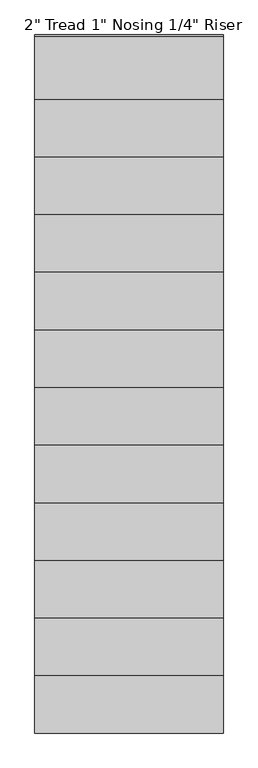
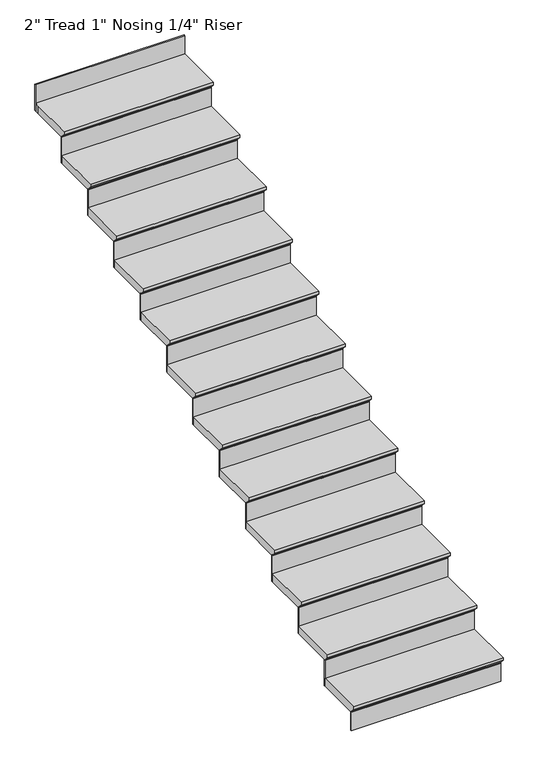
"""IFC4 building model written with IfcOpenShell, lengths in millimetres: stair flight geometry."""

from ifc_helpers import new_model, si_unit, origin, place, context, project, spatial, faceted_brep, source, transform, mapped, element, save


def stair_flight_9c09f5e7(model_context):
    return source(origin(), model_context, "Body", "Brep", [
        faceted_brep([(-2703.0415084, 19841.9216096, 37576.9005799), (-2703.0415084, 19841.9216096, 37595.9505799), (-3617.4415084, 19841.9216096, 37595.9505799), (-3617.4415084, 19841.9216096, 37576.9005799), (-2703.0415084, 19867.3216096, 37551.5005799), (-3617.4415084, 19867.3216096, 37551.5005799), (-2703.0415084, 20146.7216096, 37595.9505799), (-3617.4415084, 20146.7216096, 37595.9505799), (-3617.4415084, 19867.3216096, 37545.1505799), (-3617.4415084, 20146.7216096, 37545.1505799), (-2703.0415084, 20146.7216096, 37545.1505799), (-2703.0415084, 19867.3216096, 37545.1505799)], [[[0, 1, 2, 3]], [[4, 0, 3, 5]], [[2, 1, 6, 7]], [[8, 9, 10, 11]], [[2, 7, 9, 8, 5, 3]], [[8, 11, 4, 5]], [[6, 1, 0, 4, 11, 10]], [[7, 6, 10, 9]]]),
        faceted_brep([(-2703.0415084, 19867.3216096, 37545.1505799), (-2703.0415084, 19867.3216096, 37426.6172466), (-2703.0415084, 19873.6716096, 37426.6172466), (-2703.0415084, 19873.6716096, 37545.1505799), (-3617.4415084, 19867.3216096, 37545.1505799), (-3617.4415084, 19873.6716096, 37545.1505799), (-3617.4415084, 19873.6716096, 37426.6172466), (-3617.4415084, 19867.3216096, 37426.6172466)], [[[0, 1, 2, 3]], [[4, 5, 6, 7]], [[1, 0, 4, 7]], [[2, 1, 7, 6]], [[3, 2, 6, 5]], [[0, 3, 5, 4]]]),
        faceted_brep([(-2703.0415084, 20146.7216096, 37714.4839133), (-2703.0415084, 20146.7216096, 37545.1505799), (-2703.0415084, 20153.0716096, 37545.1505799), (-2703.0415084, 20153.0716096, 37714.4839133), (-3617.4415084, 20146.7216096, 37714.4839133), (-3617.4415084, 20153.0716096, 37714.4839133), (-3617.4415084, 20153.0716096, 37545.1505799), (-3617.4415084, 20146.7216096, 37545.1505799)], [[[0, 1, 2, 3]], [[4, 5, 6, 7]], [[1, 0, 4, 7]], [[2, 1, 7, 6]], [[3, 2, 6, 5]], [[0, 3, 5, 4]]]),
        faceted_brep([(-3617.4415084, 20121.3216096, 37765.2839133), (-2703.0415084, 20121.3216096, 37765.2839133), (-2703.0415084, 20426.1216096, 37765.2839133), (-3617.4415084, 20426.1216096, 37765.2839133), (-3617.4415084, 20146.7216096, 37714.4839133), (-3617.4415084, 20426.1216096, 37714.4839133), (-2703.0415084, 20426.1216096, 37714.4839133), (-2703.0415084, 20146.7216096, 37714.4839133), (-3617.4415084, 20146.7216096, 37720.8339133), (-3617.4415084, 20121.3216096, 37746.2339133), (-2703.0415084, 20146.7216096, 37720.8339133), (-2703.0415084, 20121.3216096, 37746.2339133)], [[[0, 1, 2, 3]], [[4, 5, 6, 7]], [[0, 3, 5, 4, 8, 9]], [[4, 7, 10, 8]], [[2, 1, 11, 10, 7, 6]], [[3, 2, 6, 5]], [[11, 1, 0, 9]], [[10, 11, 9, 8]]]),
        faceted_brep([(-2703.0415084, 20426.1216096, 37883.8172466), (-2703.0415084, 20426.1216096, 37714.4839133), (-2703.0415084, 20432.4716096, 37714.4839133), (-2703.0415084, 20432.4716096, 37883.8172466), (-3617.4415084, 20426.1216096, 37883.8172466), (-3617.4415084, 20432.4716096, 37883.8172466), (-3617.4415084, 20432.4716096, 37714.4839133), (-3617.4415084, 20426.1216096, 37714.4839133)], [[[0, 1, 2, 3]], [[4, 5, 6, 7]], [[1, 0, 4, 7]], [[2, 1, 7, 6]], [[3, 2, 6, 5]], [[0, 3, 5, 4]]]),
        faceted_brep([(-3617.4415084, 20400.7216096, 37934.6172466), (-2703.0415084, 20400.7216096, 37934.6172466), (-2703.0415084, 20705.5216096, 37934.6172466), (-3617.4415084, 20705.5216096, 37934.6172466), (-3617.4415084, 20426.1216096, 37883.8172466), (-3617.4415084, 20705.5216096, 37883.8172466), (-2703.0415084, 20705.5216096, 37883.8172466), (-2703.0415084, 20426.1216096, 37883.8172466), (-3617.4415084, 20426.1216096, 37890.1672466), (-3617.4415084, 20400.7216096, 37915.5672466), (-2703.0415084, 20426.1216096, 37890.1672466), (-2703.0415084, 20400.7216096, 37915.5672466)], [[[0, 1, 2, 3]], [[4, 5, 6, 7]], [[0, 3, 5, 4, 8, 9]], [[4, 7, 10, 8]], [[2, 1, 11, 10, 7, 6]], [[3, 2, 6, 5]], [[11, 1, 0, 9]], [[10, 11, 9, 8]]]),
        faceted_brep([(-2703.0415084, 20705.5216096, 38053.1505799), (-2703.0415084, 20705.5216096, 37883.8172466), (-2703.0415084, 20711.8716096, 37883.8172466), (-2703.0415084, 20711.8716096, 38053.1505799), (-3617.4415084, 20705.5216096, 38053.1505799), (-3617.4415084, 20711.8716096, 38053.1505799), (-3617.4415084, 20711.8716096, 37883.8172466), (-3617.4415084, 20705.5216096, 37883.8172466)], [[[0, 1, 2, 3]], [[4, 5, 6, 7]], [[1, 0, 4, 7]], [[2, 1, 7, 6]], [[3, 2, 6, 5]], [[0, 3, 5, 4]]]),
        faceted_brep([(-3617.4415084, 20680.1216096, 38103.9505799), (-2703.0415084, 20680.1216096, 38103.9505799), (-2703.0415084, 20984.9216096, 38103.9505799), (-3617.4415084, 20984.9216096, 38103.9505799), (-3617.4415084, 20705.5216096, 38053.1505799), (-3617.4415084, 20984.9216096, 38053.1505799), (-2703.0415084, 20984.9216096, 38053.1505799), (-2703.0415084, 20705.5216096, 38053.1505799), (-3617.4415084, 20705.5216096, 38059.5005799), (-3617.4415084, 20680.1216096, 38084.9005799), (-2703.0415084, 20705.5216096, 38059.5005799), (-2703.0415084, 20680.1216096, 38084.9005799)], [[[0, 1, 2, 3]], [[4, 5, 6, 7]], [[0, 3, 5, 4, 8, 9]], [[4, 7, 10, 8]], [[2, 1, 11, 10, 7, 6]], [[3, 2, 6, 5]], [[11, 1, 0, 9]], [[10, 11, 9, 8]]]),
        faceted_brep([(-2703.0415084, 20984.9216096, 38222.4839133), (-2703.0415084, 20984.9216096, 38053.1505799), (-2703.0415084, 20991.2716096, 38053.1505799), (-2703.0415084, 20991.2716096, 38222.4839133), (-3617.4415084, 20984.9216096, 38222.4839133), (-3617.4415084, 20991.2716096, 38222.4839133), (-3617.4415084, 20991.2716096, 38053.1505799), (-3617.4415084, 20984.9216096, 38053.1505799)], [[[0, 1, 2, 3]], [[4, 5, 6, 7]], [[1, 0, 4, 7]], [[2, 1, 7, 6]], [[3, 2, 6, 5]], [[0, 3, 5, 4]]]),
        faceted_brep([(-3617.4415084, 20959.5216096, 38273.2839133), (-2703.0415084, 20959.5216096, 38273.2839133), (-2703.0415084, 21264.3216096, 38273.2839133), (-3617.4415084, 21264.3216096, 38273.2839133), (-3617.4415084, 20984.9216096, 38222.4839133), (-3617.4415084, 21264.3216096, 38222.4839133), (-2703.0415084, 21264.3216096, 38222.4839133), (-2703.0415084, 20984.9216096, 38222.4839133), (-3617.4415084, 20984.9216096, 38228.8339133), (-3617.4415084, 20959.5216096, 38254.2339133), (-2703.0415084, 20984.9216096, 38228.8339133), (-2703.0415084, 20959.5216096, 38254.2339133)], [[[0, 1, 2, 3]], [[4, 5, 6, 7]], [[0, 3, 5, 4, 8, 9]], [[4, 7, 10, 8]], [[2, 1, 11, 10, 7, 6]], [[3, 2, 6, 5]], [[11, 1, 0, 9]], [[10, 11, 9, 8]]]),
        faceted_brep([(-2703.0415084, 21264.3216096, 38391.8172466), (-2703.0415084, 21264.3216096, 38222.4839133), (-2703.0415084, 21270.6716096, 38222.4839133), (-2703.0415084, 21270.6716096, 38391.8172466), (-3617.4415084, 21264.3216096, 38391.8172466), (-3617.4415084, 21270.6716096, 38391.8172466), (-3617.4415084, 21270.6716096, 38222.4839133), (-3617.4415084, 21264.3216096, 38222.4839133)], [[[0, 1, 2, 3]], [[4, 5, 6, 7]], [[1, 0, 4, 7]], [[2, 1, 7, 6]], [[3, 2, 6, 5]], [[0, 3, 5, 4]]]),
        faceted_brep([(-3617.4415084, 21238.9216096, 38442.6172466), (-2703.0415084, 21238.9216096, 38442.6172466), (-2703.0415084, 21543.7216096, 38442.6172466), (-3617.4415084, 21543.7216096, 38442.6172466), (-3617.4415084, 21264.3216096, 38391.8172466), (-3617.4415084, 21543.7216096, 38391.8172466), (-2703.0415084, 21543.7216096, 38391.8172466), (-2703.0415084, 21264.3216096, 38391.8172466), (-3617.4415084, 21264.3216096, 38398.1672466), (-3617.4415084, 21238.9216096, 38423.5672466), (-2703.0415084, 21264.3216096, 38398.1672466), (-2703.0415084, 21238.9216096, 38423.5672466)], [[[0, 1, 2, 3]], [[4, 5, 6, 7]], [[0, 3, 5, 4, 8, 9]], [[4, 7, 10, 8]], [[2, 1, 11, 10, 7, 6]], [[3, 2, 6, 5]], [[11, 1, 0, 9]], [[10, 11, 9, 8]]]),
        faceted_brep([(-2703.0415084, 21543.7216096, 38561.1505799), (-2703.0415084, 21543.7216096, 38391.8172466), (-2703.0415084, 21550.0716096, 38391.8172466), (-2703.0415084, 21550.0716096, 38561.1505799), (-3617.4415084, 21543.7216096, 38561.1505799), (-3617.4415084, 21550.0716096, 38561.1505799), (-3617.4415084, 21550.0716096, 38391.8172466), (-3617.4415084, 21543.7216096, 38391.8172466)], [[[0, 1, 2, 3]], [[4, 5, 6, 7]], [[1, 0, 4, 7]], [[2, 1, 7, 6]], [[3, 2, 6, 5]], [[0, 3, 5, 4]]]),
        faceted_brep([(-3617.4415084, 21518.3216096, 38611.9505799), (-2703.0415084, 21518.3216096, 38611.9505799), (-2703.0415084, 21823.1216096, 38611.9505799), (-3617.4415084, 21823.1216096, 38611.9505799), (-3617.4415084, 21543.7216096, 38561.1505799), (-3617.4415084, 21823.1216096, 38561.1505799), (-2703.0415084, 21823.1216096, 38561.1505799), (-2703.0415084, 21543.7216096, 38561.1505799), (-3617.4415084, 21543.7216096, 38567.5005799), (-3617.4415084, 21518.3216096, 38592.9005799), (-2703.0415084, 21543.7216096, 38567.5005799), (-2703.0415084, 21518.3216096, 38592.9005799)], [[[0, 1, 2, 3]], [[4, 5, 6, 7]], [[0, 3, 5, 4, 8, 9]], [[4, 7, 10, 8]], [[2, 1, 11, 10, 7, 6]], [[3, 2, 6, 5]], [[11, 1, 0, 9]], [[10, 11, 9, 8]]]),
        faceted_brep([(-2703.0415084, 21823.1216096, 38730.4839133), (-2703.0415084, 21823.1216096, 38561.1505799), (-2703.0415084, 21829.4716096, 38561.1505799), (-2703.0415084, 21829.4716096, 38730.4839133), (-3617.4415084, 21823.1216096, 38730.4839133), (-3617.4415084, 21829.4716096, 38730.4839133), (-3617.4415084, 21829.4716096, 38561.1505799), (-3617.4415084, 21823.1216096, 38561.1505799)], [[[0, 1, 2, 3]], [[4, 5, 6, 7]], [[1, 0, 4, 7]], [[2, 1, 7, 6]], [[3, 2, 6, 5]], [[0, 3, 5, 4]]]),
        faceted_brep([(-3617.4415084, 21797.7216096, 38781.2839133), (-2703.0415084, 21797.7216096, 38781.2839133), (-2703.0415084, 22102.5216096, 38781.2839133), (-3617.4415084, 22102.5216096, 38781.2839133), (-3617.4415084, 21823.1216096, 38730.4839133), (-3617.4415084, 22102.5216096, 38730.4839133), (-2703.0415084, 22102.5216096, 38730.4839133), (-2703.0415084, 21823.1216096, 38730.4839133), (-3617.4415084, 21823.1216096, 38736.8339133), (-3617.4415084, 21797.7216096, 38762.2339133), (-2703.0415084, 21823.1216096, 38736.8339133), (-2703.0415084, 21797.7216096, 38762.2339133)], [[[0, 1, 2, 3]], [[4, 5, 6, 7]], [[0, 3, 5, 4, 8, 9]], [[4, 7, 10, 8]], [[2, 1, 11, 10, 7, 6]], [[3, 2, 6, 5]], [[11, 1, 0, 9]], [[10, 11, 9, 8]]]),
        faceted_brep([(-2703.0415084, 22102.5216096, 38899.8172466), (-2703.0415084, 22102.5216096, 38730.4839133), (-2703.0415084, 22108.8716096, 38730.4839133), (-2703.0415084, 22108.8716096, 38899.8172466), (-3617.4415084, 22102.5216096, 38899.8172466), (-3617.4415084, 22108.8716096, 38899.8172466), (-3617.4415084, 22108.8716096, 38730.4839133), (-3617.4415084, 22102.5216096, 38730.4839133)], [[[0, 1, 2, 3]], [[4, 5, 6, 7]], [[1, 0, 4, 7]], [[2, 1, 7, 6]], [[3, 2, 6, 5]], [[0, 3, 5, 4]]]),
        faceted_brep([(-3617.4415084, 22077.1216096, 38950.6172466), (-2703.0415084, 22077.1216096, 38950.6172466), (-2703.0415084, 22381.9216096, 38950.6172466), (-3617.4415084, 22381.9216096, 38950.6172466), (-3617.4415084, 22102.5216096, 38899.8172466), (-3617.4415084, 22381.9216096, 38899.8172466), (-2703.0415084, 22381.9216096, 38899.8172466), (-2703.0415084, 22102.5216096, 38899.8172466), (-3617.4415084, 22102.5216096, 38906.1672466), (-3617.4415084, 22077.1216096, 38931.5672466), (-2703.0415084, 22102.5216096, 38906.1672466), (-2703.0415084, 22077.1216096, 38931.5672466)], [[[0, 1, 2, 3]], [[4, 5, 6, 7]], [[0, 3, 5, 4, 8, 9]], [[4, 7, 10, 8]], [[2, 1, 11, 10, 7, 6]], [[3, 2, 6, 5]], [[11, 1, 0, 9]], [[10, 11, 9, 8]]]),
        faceted_brep([(-2703.0415084, 22381.9216096, 39069.1505799), (-2703.0415084, 22381.9216096, 38899.8172466), (-2703.0415084, 22388.2716096, 38899.8172466), (-2703.0415084, 22388.2716096, 39069.1505799), (-3617.4415084, 22381.9216096, 39069.1505799), (-3617.4415084, 22388.2716096, 39069.1505799), (-3617.4415084, 22388.2716096, 38899.8172466), (-3617.4415084, 22381.9216096, 38899.8172466)], [[[0, 1, 2, 3]], [[4, 5, 6, 7]], [[1, 0, 4, 7]], [[2, 1, 7, 6]], [[3, 2, 6, 5]], [[0, 3, 5, 4]]]),
        faceted_brep([(-3617.4415084, 22356.5216096, 39119.9505799), (-2703.0415084, 22356.5216096, 39119.9505799), (-2703.0415084, 22661.3216096, 39119.9505799), (-3617.4415084, 22661.3216096, 39119.9505799), (-3617.4415084, 22381.9216096, 39069.1505799), (-3617.4415084, 22661.3216096, 39069.1505799), (-2703.0415084, 22661.3216096, 39069.1505799), (-2703.0415084, 22381.9216096, 39069.1505799), (-3617.4415084, 22381.9216096, 39075.5005799), (-3617.4415084, 22356.5216096, 39100.9005799), (-2703.0415084, 22381.9216096, 39075.5005799), (-2703.0415084, 22356.5216096, 39100.9005799)], [[[0, 1, 2, 3]], [[4, 5, 6, 7]], [[0, 3, 5, 4, 8, 9]], [[4, 7, 10, 8]], [[2, 1, 11, 10, 7, 6]], [[3, 2, 6, 5]], [[11, 1, 0, 9]], [[10, 11, 9, 8]]]),
        faceted_brep([(-2703.0415084, 22661.3216096, 39238.4839133), (-2703.0415084, 22661.3216096, 39069.1505799), (-2703.0415084, 22667.6716096, 39069.1505799), (-2703.0415084, 22667.6716096, 39238.4839133), (-3617.4415084, 22661.3216096, 39238.4839133), (-3617.4415084, 22667.6716096, 39238.4839133), (-3617.4415084, 22667.6716096, 39069.1505799), (-3617.4415084, 22661.3216096, 39069.1505799)], [[[0, 1, 2, 3]], [[4, 5, 6, 7]], [[1, 0, 4, 7]], [[2, 1, 7, 6]], [[3, 2, 6, 5]], [[0, 3, 5, 4]]]),
        faceted_brep([(-3617.4415084, 22635.9216096, 39289.2839133), (-2703.0415084, 22635.9216096, 39289.2839133), (-2703.0415084, 22940.7216096, 39289.2839133), (-3617.4415084, 22940.7216096, 39289.2839133), (-3617.4415084, 22661.3216096, 39238.4839133), (-3617.4415084, 22940.7216096, 39238.4839133), (-2703.0415084, 22940.7216096, 39238.4839133), (-2703.0415084, 22661.3216096, 39238.4839133), (-3617.4415084, 22661.3216096, 39244.8339133), (-3617.4415084, 22635.9216096, 39270.2339133), (-2703.0415084, 22661.3216096, 39244.8339133), (-2703.0415084, 22635.9216096, 39270.2339133)], [[[0, 1, 2, 3]], [[4, 5, 6, 7]], [[0, 3, 5, 4, 8, 9]], [[4, 7, 10, 8]], [[2, 1, 11, 10, 7, 6]], [[3, 2, 6, 5]], [[11, 1, 0, 9]], [[10, 11, 9, 8]]]),
        faceted_brep([(-2703.0415084, 23220.1216096, 39577.1505799), (-2703.0415084, 23220.1216096, 39407.8172466), (-2703.0415084, 23226.4716096, 39407.8172466), (-2703.0415084, 23226.4716096, 39577.1505799), (-3617.4415084, 23220.1216096, 39577.1505799), (-3617.4415084, 23226.4716096, 39577.1505799), (-3617.4415084, 23226.4716096, 39407.8172466), (-3617.4415084, 23220.1216096, 39407.8172466)], [[[0, 1, 2, 3]], [[4, 5, 6, 7]], [[1, 0, 4, 7]], [[2, 1, 7, 6]], [[3, 2, 6, 5]], [[0, 3, 5, 4]]]),
        faceted_brep([(-2703.0415084, 22940.7216096, 39407.8172466), (-2703.0415084, 22940.7216096, 39238.4839133), (-2703.0415084, 22947.0716096, 39238.4839133), (-2703.0415084, 22947.0716096, 39407.8172466), (-3617.4415084, 22940.7216096, 39407.8172466), (-3617.4415084, 22947.0716096, 39407.8172466), (-3617.4415084, 22947.0716096, 39238.4839133), (-3617.4415084, 22940.7216096, 39238.4839133)], [[[0, 1, 2, 3]], [[4, 5, 6, 7]], [[1, 0, 4, 7]], [[2, 1, 7, 6]], [[3, 2, 6, 5]], [[0, 3, 5, 4]]]),
        faceted_brep([(-3617.4415084, 23220.1216096, 39458.6172466), (-3617.4415084, 23194.7216096, 39458.6172466), (-3617.4415084, 22915.3216096, 39458.6172466), (-2703.0415084, 22915.3216096, 39458.6172466), (-2703.0415084, 23220.1216096, 39458.6172466), (-3617.4415084, 23194.7216096, 39407.8172466), (-3617.4415084, 23220.1216096, 39407.8172466), (-2703.0415084, 23220.1216096, 39407.8172466), (-2703.0415084, 22940.7216096, 39407.8172466), (-3617.4415084, 22940.7216096, 39407.8172466), (-3617.4415084, 22940.7216096, 39414.1672466), (-3617.4415084, 22915.3216096, 39439.5672466), (-2703.0415084, 22940.7216096, 39414.1672466), (-2703.0415084, 22915.3216096, 39439.5672466)], [[[0, 1, 2, 3, 4]], [[5, 6, 7, 8, 9]], [[1, 0, 6, 5]], [[2, 1, 5, 9, 10, 11]], [[9, 8, 12, 10]], [[4, 3, 13, 12, 8, 7]], [[0, 4, 7, 6]], [[13, 3, 2, 11]], [[12, 13, 11, 10]]]),
    ])


if __name__ == "__main__":
    model = new_model("IFC4")
    model_context = context("Model", 3, world=origin())
    ifc_project = project(units=[si_unit("LENGTHUNIT", "METRE", prefix="MILLI")], contexts=[model_context])
    site = spatial("IfcSite", under=ifc_project)
    building = spatial("IfcBuilding", under=site)
    placement = place(None, origin())
    stair_flight_shape = stair_flight_9c09f5e7(model_context)
    element("IfcStairFlight", 1, ObjectType="2\" Tread 1\" Nosing 1/4\" Riser", at=placement, inside=building, context=model_context, shape_type="MappedRepresentation", body=[
        mapped(stair_flight_shape, transform((0.0, 0.0, 0.0), x_axis=(1.0, 0.0, 0.0), y_axis=(0.0, 1.0, 0.0), z_axis=(0.0, 0.0, 1.0))),
    ])
    save(model, "model.ifc")
